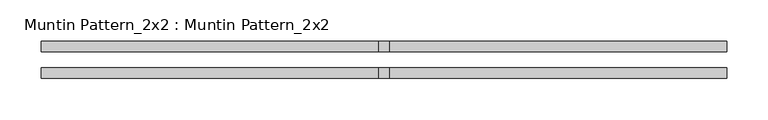
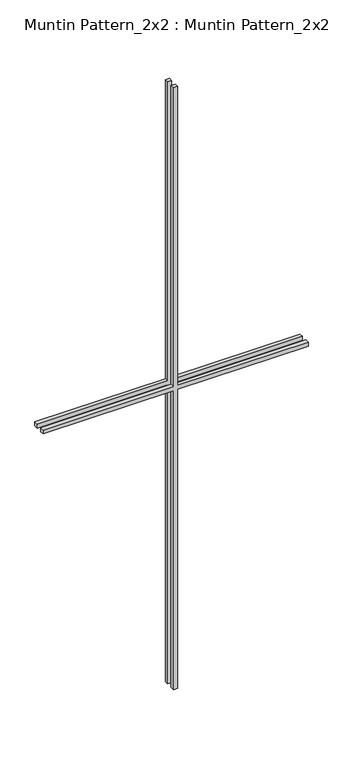
"""IFC4 building model written with IfcOpenShell, lengths in millimetres: proxy geometry, Muntin Pattern_2x2 : Muntin Pattern_2x2."""

from ifc_helpers import new_model, si_unit, frame, origin, place, context, project, spatial, polyline, outline, extrude, source, transform, mapped, element, save


def muntin_pattern_2x2_muntin_pattern_2x2_bf2b9acc(model_context):
    return source(origin(), model_context, "Body", "SweptSolid", [
        extrude(outline(polyline([(1000.125, -6.35), (1000.125, -414.3375), (987.425, -414.3375), (987.425, -6.35), (0.0, -6.35), (0.0, 6.35), (987.425, 6.35), (987.425, 414.3375), (1000.125, 414.3375), (1000.125, 6.35), (1987.55, 6.35), (1987.55, -6.35), (1000.125, -6.35)])), frame((0.0, 9.525, 0.0), z_axis=(0.0, 1.0, 0.0), x_axis=(0.0, 0.0, 1.0)), (0.0, 0.0, 1.0), 12.7),
        extrude(outline(polyline([(1000.125, -6.35), (1000.125, -414.3375), (987.425, -414.3375), (987.425, -6.35), (0.0, -6.35), (0.0, 6.35), (987.425, 6.35), (987.425, 414.3375), (1000.125, 414.3375), (1000.125, 6.35), (1987.55, 6.35), (1987.55, -6.35), (1000.125, -6.35)])), frame((0.0, -22.225, 0.0), z_axis=(0.0, 1.0, 0.0), x_axis=(0.0, 0.0, 1.0)), (0.0, 0.0, 1.0), 12.7),
    ])


if __name__ == "__main__":
    model = new_model("IFC4")
    model_context = context("Model", 3, world=origin())
    ifc_project = project(units=[si_unit("LENGTHUNIT", "METRE", prefix="MILLI")], contexts=[model_context])
    site = spatial("IfcSite", under=ifc_project)
    building = spatial("IfcBuilding", under=site)
    placement = place(None, origin())
    muntin_pattern_2x2_muntin_pattern_2x2_shape = muntin_pattern_2x2_muntin_pattern_2x2_bf2b9acc(model_context)
    element("IfcBuildingElementProxy", 1, Name="Muntin Pattern_2x2 : Muntin Pattern_2x2", ObjectType="Muntin Pattern_2x2 : Muntin Pattern_2x2", at=placement, inside=building, context=model_context, shape_type="MappedRepresentation", body=[
        mapped(muntin_pattern_2x2_muntin_pattern_2x2_shape, transform((0.0, 0.0, 0.0), x_axis=(1.0, 0.0, 0.0), y_axis=(0.0, 1.0, 0.0), z_axis=(0.0, 0.0, 1.0))),
    ])
    save(model, "model.ifc")

# Revit data of these elements
# Type "Muntin Pattern_2x2 : Muntin Pattern_2x2"
#   Width [instance default] = 4' - 0"
#   Thickness = 0' - 0 1/2"
#   Height [instance default] = 4' - 0"
#   Distance = 0' - 0 3/4"
#   Interior Material [instance default] = none
#   Exterior Material [instance default] = none
#   Default Elevation = 0
# Element 1 (IfcBuildingElementProxy, "Muntin Pattern_2x2 : Muntin Pattern_2x2")
#   Width = 2' - 8 5/8"
#   Height = 6' - 6 1/4"
#   Interior Material = Wood - Stained
#   Exterior Material = Clad - White
#   Materials on its faces: "Clad - White", "Wood - Stained"
# Materials
#   "Clad - White": class "Wood", colour RGB 242 242 238, transparency 0, Cost = 0
#   "Wood - Stained": class "Wood", colour RGB 224 178 126, transparency 0, Cost = 0
